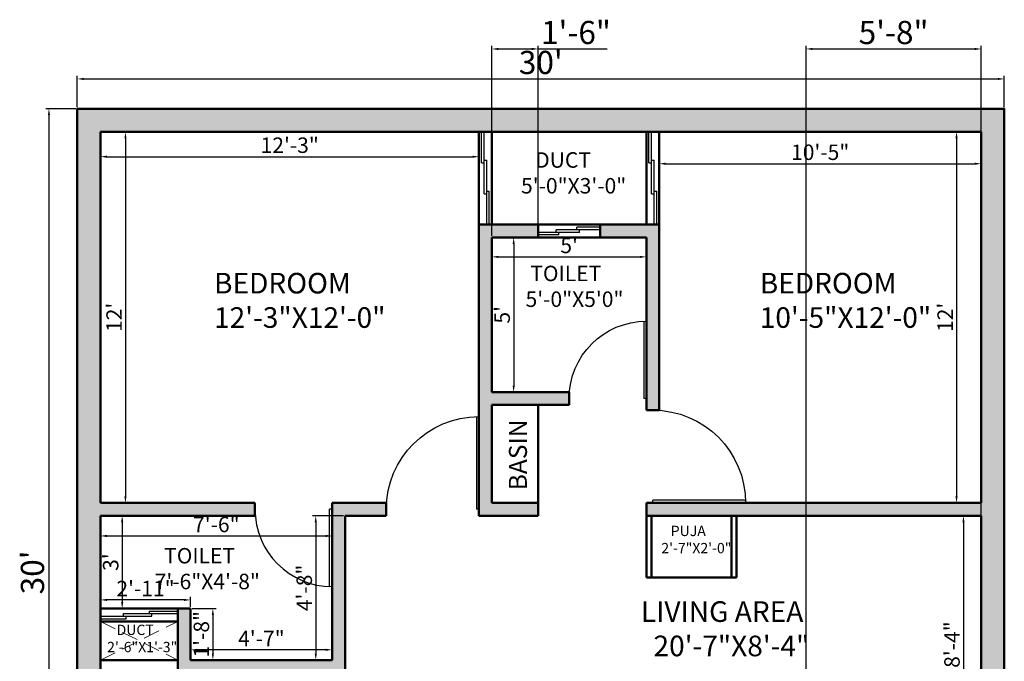
# Model space of a CAD drawing. Units: inches. Extents: x 3274 to 5176, y 1085 to 2172.
# Tile 2 of 16: x 3351 to 3733, y 1325 to 1574. Entities that reach past the tile are written whole.
import ezdxf

# ---------------------------------------------------------------- set-up
doc = ezdxf.new("R2010")
doc.units = ezdxf.units.IN
doc.linetypes.add('DASHED', pattern=[19.05, 12.7, -6.35])
for name, color, linetype, lineweight in [('A-ANNO-DIMS', 2, 'Continuous', 18), ('A-AREA-IDEN', 3, 'Continuous', 25), ('A-DOOR', 4, 'Continuous', 25), ('A-FLOR-OPEN', 7, 'DASHED', 18), ('A-GLAZ', 5, 'Continuous', 25), ('A-WALL', 7, 'Continuous', 50), ('A-WALL-PATT', 8, 'Continuous', 13)]:
    doc.layers.add(name, color=color, linetype=linetype, lineweight=lineweight)
doc.styles.get("Standard").update_dxf_attribs({"font": 'arial.ttf'})
doc.dimstyles.new('ISO-25', dxfattribs={"dimtxt": 9, "dimasz": 2.5, "dimexe": 1.25, "dimexo": 0.625, "dimtad": 1, "dimdec": 1, "dimlunit": 3, "dimtxsty": 'Standard', "dimcen": 2.5, "dimclrd": 4, "dimclre": 4, "dimclrt": 1, "dimadec": 0, "dimazin": 0, "dimtfac": 1, "dimtdec": 1, "dimtmove": 0, "dimatfit": 3, "dimfxl": 1, "dimarcsym": 0})

# ---------------------------------------------------------------- blocks, each defined once
blk = doc.blocks.new('1')
for p, q in [((0, 36), (0, 0)), ((1, 36), (1, 0)), ((0, 0), (1, 0))]:
    blk.add_line(p, q)
blk.add_arc((0, 0), 36, 0, 90)
blk = doc.blocks.new('2')
for p, q in [((0, 30), (0, 0)), ((1, 30), (1, 0)), ((0, 0), (1, 0))]:
    blk.add_line(p, q)
blk.add_arc((0, 0), 30, 0, 90)
blk = doc.blocks.new('*D10')
at = {"layer": 'A-ANNO-DIMS', "color": 0, "lineweight": -2, "transparency": 16777216}
for p, q in [((3373.3, 1539.91), (3373.3, 1552.09)), ((3375.8, 1550.84), (3730.8, 1550.84)), ((3733.3, 1539.91), (3733.3, 1552.09))]:
    blk.add_line(p, q, dxfattribs=at)
at = {"layer": 'A-ANNO-DIMS', "color": 0, "transparency": 16777216}
for points in [[(3375.8, 1551.26), (3375.8, 1550.43), (3373.3, 1550.84)], [(3730.8, 1551.26), (3730.8, 1550.43), (3733.3, 1550.84)]]:
    blk.add_solid(points, dxfattribs=at)
at = {"layer": 'Defpoints', "color": 0, "transparency": 16777216}
for p in [(3733.3, 1550.84), (3373.3, 1539.28), (3733.3, 1539.28)]:
    blk.add_point(p, dxfattribs=at)
at = {"layer": 'A-ANNO-DIMS', "color": 0, "transparency": 16777216, "insert": (3553.3, 1556.07), "char_height": 9, "attachment_point": 5}
blk.add_mtext("30'", dxfattribs=at)
blk = doc.blocks.new('*D11')
at = {"layer": 'A-ANNO-DIMS', "color": 0, "lineweight": -2, "transparency": 16777216}
for p, q in [((3372.68, 1539.28), (3361.05, 1539.28)), ((3362.3, 1536.78), (3362.3, 1181.78)), ((3372.68, 1179.28), (3361.05, 1179.28))]:
    blk.add_line(p, q, dxfattribs=at)
at = {"layer": 'A-ANNO-DIMS', "color": 0, "transparency": 16777216}
for points in [[(3361.88, 1536.78), (3362.71, 1536.78), (3362.3, 1539.28)], [(3361.88, 1181.78), (3362.71, 1181.78), (3362.3, 1179.28)]]:
    blk.add_solid(points, dxfattribs=at)
at = {"layer": 'Defpoints', "color": 0, "transparency": 16777216}
for p in [(3373.3, 1539.28), (3362.3, 1179.28), (3373.3, 1179.28)]:
    blk.add_point(p, dxfattribs=at)
at = {"layer": 'A-ANNO-DIMS', "color": 0, "transparency": 16777216, "insert": (3357.07, 1359.28), "char_height": 9, "attachment_point": 5, "rotation": 90}
blk.add_mtext("30'", dxfattribs=at)
blk = doc.blocks.new('*D12')
at = {"layer": 'A-ANNO-DIMS', "color": 0, "lineweight": -2, "transparency": 16777216}
for p, q in [((3382.3, 1529.66), (3382.3, 1519.4)), ((3529.3, 1529.66), (3529.3, 1519.4)), ((3384.8, 1520.65), (3526.8, 1520.65))]:
    blk.add_line(p, q, dxfattribs=at)
at = {"layer": 'A-ANNO-DIMS', "color": 0, "transparency": 16777216}
for points in [[(3384.8, 1521.07), (3384.8, 1520.24), (3382.3, 1520.65)], [(3526.8, 1521.07), (3526.8, 1520.24), (3529.3, 1520.65)]]:
    blk.add_solid(points, dxfattribs=at)
at = {"layer": 'Defpoints', "color": 0, "transparency": 16777216}
for p in [(3382.3, 1530.28), (3529.3, 1530.28), (3529.3, 1520.65)]:
    blk.add_point(p, dxfattribs=at)
at = {"layer": 'A-ANNO-DIMS', "color": 0, "transparency": 16777216, "insert": (3455.8, 1524.34), "char_height": 6, "attachment_point": 5}
blk.add_mtext('12\'-3"', dxfattribs=at)
blk = doc.blocks.new('*D13')
at = {"layer": 'A-ANNO-DIMS', "color": 0, "lineweight": -2, "transparency": 16777216}
for p, q in [((3382.93, 1530.28), (3393.26, 1530.28)), ((3392.01, 1527.78), (3392.01, 1388.78)), ((3382.93, 1386.28), (3393.26, 1386.28))]:
    blk.add_line(p, q, dxfattribs=at)
at = {"layer": 'A-ANNO-DIMS', "color": 0, "transparency": 16777216}
for points in [[(3391.59, 1527.78), (3392.42, 1527.78), (3392.01, 1530.28)], [(3391.59, 1388.78), (3392.42, 1388.78), (3392.01, 1386.28)]]:
    blk.add_solid(points, dxfattribs=at)
at = {"layer": 'Defpoints', "color": 0, "transparency": 16777216}
for p in [(3382.3, 1530.28), (3382.3, 1386.28), (3392.01, 1386.28)]:
    blk.add_point(p, dxfattribs=at)
at = {"layer": 'A-ANNO-DIMS', "color": 0, "transparency": 16777216, "insert": (3388.37, 1458.28), "char_height": 6, "attachment_point": 5, "rotation": 90}
blk.add_mtext("12'", dxfattribs=at)
blk = doc.blocks.new('*D14')
at = {"layer": 'A-ANNO-DIMS', "color": 0, "lineweight": -2, "transparency": 16777216}
for p, q in [((3417.3, 1325.91), (3417.3, 1330.49)), ((3469.8, 1329.24), (3419.8, 1329.24)), ((3472.3, 1325.91), (3472.3, 1330.49))]:
    blk.add_line(p, q, dxfattribs=at)
at = {"layer": 'A-ANNO-DIMS', "color": 0, "transparency": 16777216}
for points in [[(3419.8, 1329.65), (3419.8, 1328.82), (3417.3, 1329.24)], [(3469.8, 1329.65), (3469.8, 1328.82), (3472.3, 1329.24)]]:
    blk.add_solid(points, dxfattribs=at)
at = {"layer": 'Defpoints', "color": 0, "transparency": 16777216}
for p in [(3417.3, 1329.24), (3417.3, 1325.28), (3472.3, 1325.28)]:
    blk.add_point(p, dxfattribs=at)
at = {"layer": 'A-ANNO-DIMS', "color": 0, "transparency": 16777216, "insert": (3444.8, 1332.86), "char_height": 6, "attachment_point": 5}
blk.add_mtext('4\'-7"', dxfattribs=at)
blk = doc.blocks.new('*D15')
at = {"layer": 'A-ANNO-DIMS', "color": 0, "lineweight": -2, "transparency": 16777216}
for p, q in [((3382.93, 1381.28), (3391.99, 1381.28)), ((3390.74, 1378.78), (3390.74, 1347.78)), ((3382.93, 1345.28), (3391.99, 1345.28))]:
    blk.add_line(p, q, dxfattribs=at)
at = {"layer": 'A-ANNO-DIMS', "color": 0, "transparency": 16777216}
for points in [[(3390.32, 1378.78), (3391.16, 1378.78), (3390.74, 1381.28)], [(3390.32, 1347.78), (3391.16, 1347.78), (3390.74, 1345.28)]]:
    blk.add_solid(points, dxfattribs=at)
at = {"layer": 'Defpoints', "color": 0, "transparency": 16777216}
for p in [(3382.3, 1381.28), (3382.3, 1345.28), (3390.74, 1345.28)]:
    blk.add_point(p, dxfattribs=at)
at = {"layer": 'A-ANNO-DIMS', "color": 0, "transparency": 16777216, "insert": (3387.05, 1363.28), "char_height": 6, "attachment_point": 5, "rotation": 90}
blk.add_mtext("3'", dxfattribs=at)
blk = doc.blocks.new('*D16')
at = {"layer": 'A-ANNO-DIMS', "color": 0, "lineweight": -2, "transparency": 16777216}
for p, q in [((3382.3, 1380.66), (3382.3, 1372.19)), ((3472.3, 1380.66), (3472.3, 1372.19)), ((3384.8, 1373.44), (3469.8, 1373.44))]:
    blk.add_line(p, q, dxfattribs=at)
at = {"layer": 'A-ANNO-DIMS', "color": 0, "transparency": 16777216}
for points in [[(3384.8, 1373.86), (3384.8, 1373.02), (3382.3, 1373.44)], [(3469.8, 1373.86), (3469.8, 1373.02), (3472.3, 1373.44)]]:
    blk.add_solid(points, dxfattribs=at)
at = {"layer": 'Defpoints', "color": 0, "transparency": 16777216}
for p in [(3382.3, 1381.28), (3472.3, 1381.28), (3472.3, 1373.44)]:
    blk.add_point(p, dxfattribs=at)
at = {"layer": 'A-ANNO-DIMS', "color": 0, "transparency": 16777216, "insert": (3427.3, 1377.13), "char_height": 6, "attachment_point": 5}
blk.add_mtext('7\'-6"', dxfattribs=at)
blk = doc.blocks.new('*D17')
at = {"layer": 'A-ANNO-DIMS', "color": 0, "lineweight": -2, "transparency": 16777216}
for p, q in [((3417.93, 1345.28), (3427.21, 1345.28)), ((3425.96, 1342.78), (3425.96, 1327.78)), ((3417.93, 1325.28), (3427.21, 1325.28))]:
    blk.add_line(p, q, dxfattribs=at)
at = {"layer": 'A-ANNO-DIMS', "color": 0, "transparency": 16777216}
for points in [[(3425.54, 1342.78), (3426.37, 1342.78), (3425.96, 1345.28)], [(3425.54, 1327.78), (3426.37, 1327.78), (3425.96, 1325.28)]]:
    blk.add_solid(points, dxfattribs=at)
at = {"layer": 'Defpoints', "color": 0, "transparency": 16777216}
for p in [(3417.3, 1345.28), (3417.3, 1325.28), (3425.96, 1325.28)]:
    blk.add_point(p, dxfattribs=at)
at = {"layer": 'A-ANNO-DIMS', "color": 0, "transparency": 16777216, "insert": (3422.27, 1335.28), "char_height": 6, "attachment_point": 5, "rotation": 90}
blk.add_mtext('1\'-8"', dxfattribs=at)
blk = doc.blocks.new('*D18')
at = {"layer": 'A-ANNO-DIMS', "color": 0, "lineweight": -2, "transparency": 16777216}
for p, q in [((3382.3, 1345.91), (3382.3, 1349.86)), ((3417.3, 1345.91), (3417.3, 1349.86)), ((3414.8, 1348.61), (3384.8, 1348.61))]:
    blk.add_line(p, q, dxfattribs=at)
at = {"layer": 'A-ANNO-DIMS', "color": 0, "transparency": 16777216}
for points in [[(3384.8, 1349.02), (3384.8, 1348.19), (3382.3, 1348.61)], [(3414.8, 1349.02), (3414.8, 1348.19), (3417.3, 1348.61)]]:
    blk.add_solid(points, dxfattribs=at)
at = {"layer": 'Defpoints', "color": 0, "transparency": 16777216}
for p in [(3382.3, 1348.61), (3382.3, 1345.28), (3417.3, 1345.28)]:
    blk.add_point(p, dxfattribs=at)
at = {"layer": 'A-ANNO-DIMS', "color": 0, "transparency": 16777216, "insert": (3399.8, 1352.24), "char_height": 6, "attachment_point": 5}
blk.add_mtext('2\'-11"', dxfattribs=at)
blk = doc.blocks.new('*D19')
at = {"layer": 'A-ANNO-DIMS', "color": 0, "lineweight": -2, "transparency": 16777216}
for p, q in [((3476.68, 1381.28), (3464.66, 1381.28)), ((3465.91, 1378.78), (3465.91, 1327.78)), ((3471.68, 1325.28), (3464.66, 1325.28))]:
    blk.add_line(p, q, dxfattribs=at)
at = {"layer": 'A-ANNO-DIMS', "color": 0, "transparency": 16777216}
for points in [[(3465.5, 1378.78), (3466.33, 1378.78), (3465.91, 1381.28)], [(3465.5, 1327.78), (3466.33, 1327.78), (3465.91, 1325.28)]]:
    blk.add_solid(points, dxfattribs=at)
at = {"layer": 'Defpoints', "color": 0, "transparency": 16777216}
for p in [(3477.3, 1381.28), (3465.91, 1325.28), (3472.3, 1325.28)]:
    blk.add_point(p, dxfattribs=at)
at = {"layer": 'A-ANNO-DIMS', "color": 0, "transparency": 16777216, "insert": (3462.22, 1353.28), "char_height": 6, "attachment_point": 5, "rotation": 90}
blk.add_mtext('4\'-8"', dxfattribs=at)
blk = doc.blocks.new('*D28')
at = {"layer": 'A-ANNO-DIMS', "color": 0, "lineweight": -2, "transparency": 16777216}
for p, q in [((3723.68, 1381.28), (3716.2, 1381.28)), ((3717.45, 1378.78), (3717.45, 1283.78)), ((3723.68, 1281.28), (3716.2, 1281.28))]:
    blk.add_line(p, q, dxfattribs=at)
at = {"layer": 'A-ANNO-DIMS', "color": 0, "transparency": 16777216}
for points in [[(3717.03, 1378.78), (3717.86, 1378.78), (3717.45, 1381.28)], [(3717.03, 1283.78), (3717.86, 1283.78), (3717.45, 1281.28)]]:
    blk.add_solid(points, dxfattribs=at)
at = {"layer": 'Defpoints', "color": 0, "transparency": 16777216}
for p in [(3724.3, 1381.28), (3717.45, 1281.28), (3724.3, 1281.28)]:
    blk.add_point(p, dxfattribs=at)
at = {"layer": 'A-ANNO-DIMS', "color": 0, "transparency": 16777216, "insert": (3713.76, 1331.28), "char_height": 6, "attachment_point": 5, "rotation": 90}
blk.add_mtext('8\'-4"', dxfattribs=at)
blk = doc.blocks.new('*D30')
at = {"layer": 'A-ANNO-DIMS', "color": 0, "lineweight": -2, "transparency": 16777216}
for p, q in [((3599.3, 1529.66), (3599.3, 1516.67)), ((3724.3, 1529.66), (3724.3, 1516.67)), ((3601.8, 1517.92), (3721.8, 1517.92))]:
    blk.add_line(p, q, dxfattribs=at)
at = {"layer": 'A-ANNO-DIMS', "color": 0, "transparency": 16777216}
for points in [[(3601.8, 1518.34), (3601.8, 1517.51), (3599.3, 1517.92)], [(3721.8, 1518.34), (3721.8, 1517.51), (3724.3, 1517.92)]]:
    blk.add_solid(points, dxfattribs=at)
at = {"layer": 'Defpoints', "color": 0, "transparency": 16777216}
for p in [(3599.3, 1530.28), (3724.3, 1530.28), (3724.3, 1517.92)]:
    blk.add_point(p, dxfattribs=at)
at = {"layer": 'A-ANNO-DIMS', "color": 0, "transparency": 16777216, "insert": (3661.8, 1521.61), "char_height": 6, "attachment_point": 5}
blk.add_mtext('10\'-5"', dxfattribs=at)
blk = doc.blocks.new('*D31')
at = {"layer": 'A-ANNO-DIMS', "color": 0, "lineweight": -2, "transparency": 16777216}
for p, q in [((3723.68, 1530.28), (3713.49, 1530.28)), ((3714.74, 1527.78), (3714.74, 1388.78)), ((3723.68, 1386.28), (3713.49, 1386.28))]:
    blk.add_line(p, q, dxfattribs=at)
at = {"layer": 'A-ANNO-DIMS', "color": 0, "transparency": 16777216}
for points in [[(3714.32, 1527.78), (3715.16, 1527.78), (3714.74, 1530.28)], [(3714.32, 1388.78), (3715.16, 1388.78), (3714.74, 1386.28)]]:
    blk.add_solid(points, dxfattribs=at)
at = {"layer": 'Defpoints', "color": 0, "transparency": 16777216}
for p in [(3724.3, 1530.28), (3714.74, 1386.28), (3724.3, 1386.28)]:
    blk.add_point(p, dxfattribs=at)
at = {"layer": 'A-ANNO-DIMS', "color": 0, "transparency": 16777216, "insert": (3711.1, 1458.28), "char_height": 6, "attachment_point": 5, "rotation": 90}
blk.add_mtext("12'", dxfattribs=at)
blk = doc.blocks.new('*D32')
at = {"layer": 'A-ANNO-DIMS', "color": 0, "lineweight": -2, "transparency": 16777216}
for p, q in [((3534.3, 1488.66), (3534.3, 1480.52)), ((3594.3, 1488.66), (3594.3, 1480.52)), ((3536.8, 1481.77), (3591.8, 1481.77))]:
    blk.add_line(p, q, dxfattribs=at)
at = {"layer": 'A-ANNO-DIMS', "color": 0, "transparency": 16777216}
for points in [[(3536.8, 1482.18), (3536.8, 1481.35), (3534.3, 1481.77)], [(3591.8, 1482.18), (3591.8, 1481.35), (3594.3, 1481.77)]]:
    blk.add_solid(points, dxfattribs=at)
at = {"layer": 'Defpoints', "color": 0, "transparency": 16777216}
for p in [(3534.3, 1489.28), (3594.3, 1489.28), (3594.3, 1481.77)]:
    blk.add_point(p, dxfattribs=at)
at = {"layer": 'A-ANNO-DIMS', "color": 0, "transparency": 16777216, "insert": (3564.3, 1485.44), "char_height": 6, "attachment_point": 5}
blk.add_mtext("5'", dxfattribs=at)
blk = doc.blocks.new('*D33')
at = {"layer": 'A-ANNO-DIMS', "color": 0, "lineweight": -2, "transparency": 16777216}
for p, q in [((3534.93, 1489.28), (3544.02, 1489.28)), ((3542.77, 1486.78), (3542.77, 1431.78)), ((3534.93, 1429.28), (3544.02, 1429.28))]:
    blk.add_line(p, q, dxfattribs=at)
at = {"layer": 'A-ANNO-DIMS', "color": 0, "transparency": 16777216}
for points in [[(3542.35, 1486.78), (3543.18, 1486.78), (3542.77, 1489.28)], [(3542.35, 1431.78), (3543.18, 1431.78), (3542.77, 1429.28)]]:
    blk.add_solid(points, dxfattribs=at)
at = {"layer": 'Defpoints', "color": 0, "transparency": 16777216}
for p in [(3534.3, 1489.28), (3534.3, 1429.28), (3542.77, 1429.28)]:
    blk.add_point(p, dxfattribs=at)
at = {"layer": 'A-ANNO-DIMS', "color": 0, "transparency": 16777216, "insert": (3539.09, 1459.28), "char_height": 6, "attachment_point": 5, "rotation": 90}
blk.add_mtext("5'", dxfattribs=at)
blk = doc.blocks.new('WIN-24')
for p, q in [((4552.19, 1485.35), (4536.19, 1485.35)), ((4544.19, 1484.35), (4536.19, 1484.35)), ((4560.19, 1486.35), (4543.19, 1486.35)), ((4543.19, 1485.35), (4543.19, 1486.35)), ((4544.19, 1484.35), (4544.19, 1485.35)), ((4551.19, 1486.35), (4551.19, 1487.35)), ((4560.19, 1487.35), (4551.19, 1487.35)), ((4552.19, 1485.35), (4552.19, 1486.35))]:
    blk.add_line(p, q)
blk = doc.blocks.new('WIN-30')
for p, q in [((4366.19, 1316.35), (4386.19, 1316.35)), ((4366.19, 1315.35), (4376.19, 1315.35)), ((4375.19, 1317.35), (4396.19, 1317.35)), ((4375.19, 1316.35), (4375.19, 1317.35)), ((4376.19, 1315.35), (4376.19, 1316.35)), ((4385.19, 1318.35), (4396.19, 1318.35)), ((4385.19, 1317.35), (4385.19, 1318.35)), ((4386.19, 1316.35), (4386.19, 1317.35))]:
    blk.add_line(p, q)
blk = doc.blocks.new('WIN-36')
for p, q in [((4514.19, 1512.35), (4514.19, 1524.35)), ((4515.19, 1500.35), (4515.19, 1524.35)), ((4514.19, 1512.35), (4515.19, 1512.35)), ((4515.19, 1513.35), (4516.19, 1513.35)), ((4516.19, 1488.35), (4516.19, 1513.35)), ((4515.19, 1500.35), (4516.19, 1500.35)), ((4516.19, 1501.35), (4517.19, 1501.35)), ((4517.19, 1488.35), (4517.19, 1501.35))]:
    blk.add_line(p, q)
blk = doc.blocks.new('*D166')
at = {"layer": 'A-ANNO-DIMS', "color": 4, "lineweight": -2, "transparency": 16777216}
for p, q in [((3656.3, 1281.91), (3656.3, 1563.73)), ((3658.8, 1562.48), (3721.8, 1562.48)), ((3724.3, 1281.91), (3724.3, 1563.73))]:
    blk.add_line(p, q, dxfattribs=at)
at = {"layer": 'A-ANNO-DIMS', "color": 4, "transparency": 16777216}
for points in [[(3658.8, 1562.9), (3658.8, 1562.06), (3656.3, 1562.48)], [(3721.8, 1562.9), (3721.8, 1562.06), (3724.3, 1562.48)]]:
    blk.add_solid(points, dxfattribs=at)
at = {"layer": 'Defpoints', "color": 0, "transparency": 16777216}
for p in [(3724.3, 1562.48), (3656.3, 1281.28), (3724.3, 1281.28)]:
    blk.add_point(p, dxfattribs=at)
at = {"layer": 'A-ANNO-DIMS', "color": 1, "transparency": 16777216, "insert": (3690.3, 1567.7), "char_height": 9, "attachment_point": 5}
blk.add_mtext('5\'-8"', dxfattribs=at)
blk = doc.blocks.new('*D167')
at = {"layer": 'A-ANNO-DIMS', "color": 4, "lineweight": -2, "transparency": 16777216}
for p, q in [((3534.3, 1489.91), (3534.3, 1563.73)), ((3536.8, 1562.48), (3549.8, 1562.48)), ((3552.3, 1489.91), (3552.3, 1563.73)), ((3552.3, 1562.48), (3579.13, 1562.48))]:
    blk.add_line(p, q, dxfattribs=at)
at = {"layer": 'A-ANNO-DIMS', "color": 4, "transparency": 16777216}
for points in [[(3536.8, 1562.9), (3536.8, 1562.06), (3534.3, 1562.48)], [(3549.8, 1562.9), (3549.8, 1562.06), (3552.3, 1562.48)]]:
    blk.add_solid(points, dxfattribs=at)
at = {"layer": 'Defpoints', "color": 0, "transparency": 16777216}
for p in [(3552.3, 1562.48), (3534.3, 1489.28), (3552.3, 1489.28)]:
    blk.add_point(p, dxfattribs=at)
at = {"layer": 'A-ANNO-DIMS', "color": 1, "transparency": 16777216, "insert": (3566.96, 1567.7), "char_height": 9, "attachment_point": 5}
blk.add_mtext('1\'-6"', dxfattribs=at)

msp = doc.modelspace()

# ---------------------------------------------------------------- hatches: boundary and pattern name
at = {"layer": 'A-WALL-PATT'}
h = msp.add_hatch(color=256, dxfattribs=at)
h.dxf.hatch_style = 1
h.paths.add_polyline_path([(3733.3, 1539.28), (3373.3, 1539.28), (3373.3, 1179.28), (3406.3, 1179.28), (3406.3, 1188.28), (3382.3, 1188.28), (3382.3, 1272.28), (3442.3, 1272.28), (3442.3, 1277.28), (3382.3, 1277.28), (3382.3, 1381.28), (3442.3, 1381.28), (3442.3, 1386.28), (3382.3, 1386.28), (3382.3, 1530.28), (3724.3, 1530.28), (3724.3, 1386.28), (3594.3, 1386.28), (3594.3, 1381.28), (3724.3, 1381.28), (3724.3, 1281.28), (3656.3, 1281.28), (3656.3, 1272.28), (3724.3, 1272.28), (3724.3, 1188.28), (3682.3, 1188.28), (3682.3, 1179.28), (3733.3, 1179.28)])
h.paths.add_polyline_path([(3477.3, 1381.28), (3493.3, 1381.28), (3493.3, 1386.28), (3472.3, 1386.28), (3472.3, 1325.28), (3417.3, 1325.28), (3417.3, 1345.28), (3412.3, 1345.28), (3412.3, 1320.28), (3472.3, 1320.28), (3472.3, 1272.28), (3493.3, 1272.28), (3493.3, 1277.28), (3477.3, 1277.28)], flags=17)
h.paths.add_polyline_path([(3534.3, 1489.28), (3552.3, 1489.28), (3552.3, 1494.28), (3529.3, 1494.28), (3529.3, 1381.28), (3552.3, 1381.28), (3552.3, 1386.28), (3534.3, 1386.28), (3534.3, 1424.28), (3564.3, 1424.28), (3564.3, 1429.28), (3534.3, 1429.28)], flags=17)
h.paths.add_polyline_path([(3599.3, 1494.28), (3576.3, 1494.28), (3576.3, 1489.28), (3594.3, 1489.28), (3594.3, 1422.28), (3599.3, 1422.28)], flags=17)
h.paths.add_polyline_path([(3534.3, 1272.28), (3539.3, 1272.28), (3539.3, 1281.28), (3529.3, 1281.28), (3529.3, 1188.28), (3478.3, 1188.28), (3478.3, 1179.28), (3534.3, 1179.28)], flags=17)
h.paths.add_polyline_path([(3596.3, 1281.28), (3587.3, 1281.28), (3587.3, 1276.78), (3587.3, 1272.28), (3596.3, 1272.28)], flags=17)
h.paths.add_polyline_path([(3610.3, 1188.28), (3594.3, 1188.28), (3594.3, 1179.28), (3610.3, 1179.28)], flags=17)
h.paths.add_polyline_path([(3589.35, 1322.21), (3663.55, 1322.21), (3663.55, 1352.06), (3589.35, 1352.06)], flags=25)
h.paths.add_polyline_path([(3545.54, 1458.93), (3584.72, 1458.93), (3584.72, 1481.32), (3545.54, 1481.32)], flags=25)
h.paths.add_polyline_path([(3635.11, 1449.68), (3703.51, 1449.68), (3703.51, 1479.54), (3635.11, 1479.54)], flags=25)
h.paths.add_polyline_path([(3543.78, 1502.97), (3585.75, 1502.97), (3585.75, 1525.36), (3543.78, 1525.36)], flags=25)
h.paths.add_polyline_path([(3423.19, 1449.68), (3491.58, 1449.68), (3491.58, 1479.54), (3423.19, 1479.54)], flags=25)

# ---------------------------------------------------------------- linework, layer by layer
at = {"layer": 'A-FLOR-OPEN', "ltscale": 0.5}
for p, q in [((3382.3, 1340.28), (3412.3, 1325.28)), ((3382.3, 1325.28), (3412.3, 1340.28))]:
    msp.add_line(p, q, dxfattribs=at)
at = {"layer": 'A-WALL'}
for p, q in [((3382.3, 1530.28), (3724.3, 1530.28)), ((3382.3, 1386.28), (3382.3, 1530.28)), ((3529.3, 1381.28), (3529.3, 1530.28)), ((3534.3, 1494.28), (3534.3, 1530.28)), ((3594.3, 1530.28), (3594.3, 1494.28)), ((3599.3, 1530.28), (3599.3, 1422.28)), ((3724.3, 1530.28), (3724.3, 1386.28)), ((3529.3, 1494.28), (3599.3, 1494.28)), ((3552.3, 1489.28), (3552.3, 1494.28)), ((3576.3, 1489.28), (3576.3, 1494.28)), ((3534.3, 1489.28), (3594.3, 1489.28)), ((3534.3, 1429.28), (3534.3, 1489.28)), ((3594.3, 1489.28), (3594.3, 1422.28)), ((3534.3, 1429.28), (3564.3, 1429.28)), ((3564.3, 1429.28), (3564.3, 1424.28)), ((3534.3, 1424.28), (3564.3, 1424.28)), ((3534.3, 1386.28), (3534.3, 1424.28)), ((3552.3, 1381.28), (3552.3, 1424.28)), ((3594.3, 1422.28), (3599.3, 1422.28)), ((3382.3, 1386.28), (3442.3, 1386.28)), ((3442.3, 1381.28), (3442.3, 1386.28)), ((3472.3, 1386.28), (3493.3, 1386.28)), ((3472.3, 1325.28), (3472.3, 1386.28)), ((3493.3, 1381.28), (3493.3, 1386.28)), ((3534.3, 1386.28), (3552.3, 1386.28)), ((3594.3, 1386.28), (3724.3, 1386.28)), ((3594.3, 1386.28), (3594.3, 1357.28)), ((3382.3, 1381.28), (3442.3, 1381.28)), ((3382.3, 1277.28), (3382.3, 1381.28)), ((3477.3, 1381.28), (3493.3, 1381.28)), ((3477.3, 1277.28), (3477.3, 1381.28)), ((3529.3, 1381.28), (3552.3, 1381.28)), ((3594.3, 1381.28), (3724.3, 1381.28)), ((3596.3, 1381.28), (3596.3, 1357.28)), ((3627.3, 1381.28), (3627.3, 1357.28)), ((3629.3, 1381.28), (3629.3, 1357.28)), ((3724.3, 1381.28), (3724.3, 1281.28)), ((3594.3, 1357.28), (3629.3, 1357.28)), ((3382.3, 1345.28), (3417.3, 1345.28)), ((3412.3, 1320.28), (3412.3, 1345.28)), ((3417.3, 1325.28), (3417.3, 1345.28)), ((3382.3, 1340.28), (3412.3, 1340.28)), ((3382.3, 1325.28), (3412.3, 1325.28)), ((3417.3, 1325.28), (3472.3, 1325.28))]:
    msp.add_line(p, q, dxfattribs=at)
msp.add_lwpolyline([(3534.3, 1179.28), (3373.3, 1179.28), (3373.3, 1539.28), (3733.3, 1539.28), (3733.3, 1179.28), (3594.3, 1179.28)], dxfattribs=at)

# ---------------------------------------------------------------- block references
at = {"layer": 'A-DOOR', "xscale": -1}
for name, p in [('2', (3594.3, 1426.78)), ('1', (3529.3, 1383.78))]:
    msp.add_blockref(name, p, dxfattribs=at)
at = {"layer": 'A-DOOR', "xscale": -1, "rotation": 270}
msp.add_blockref('1', (3596.8, 1386.28), dxfattribs=at)
at = {"layer": 'A-DOOR', "rotation": 180}
msp.add_blockref('2', (3472.3, 1383.78), dxfattribs=at)
at = {"layer": 'A-GLAZ'}
for name, p in [('WIN-36', (-983.89, 5.93)), ('WIN-36', (-918.89, 5.93)), ('WIN-24', (-983.89, 5.93)), ('WIN-30', (-983.89, 25.93))]:
    msp.add_blockref(name, p, dxfattribs=at)

# ---------------------------------------------------------------- texts
at = {"layer": 'A-AREA-IDEN', "attachment_point": 1}
for s, width, heights, insert, char_height in [('   DUCT\\P5\'-0"X3\'-0"', 58.0121, [16.24], (3545.63, 1522.37), 6), (' TOILET\\P5\'-0"X5\'0"', 58.0121, [0], (3547.39, 1478.34), 6), ('BEDROOM\\P12\'-3"X12\'-0"', 58.0121, [0], (3426.41, 1475.56), 8), ('BEDROOM\\P10\'-5"X12\'-0"', 58.0121, [0], (3638.33, 1475.56), 8), ('   PUJA\\P2\'-7"X2\'-0"', 58.0121, [16.24], (3600.1, 1377.39), 4), ('  TOILET\\P7\'-6"X4\'-8"', 58.0121, [16.24], (3403.37, 1368.76), 6), ('LIVING AREA\\P  20\'-7"X8\'-4"', 90.1483, [0], (3592.17, 1348.08), 8), ('   DUCT\\P2\'-6"X1\'-3"', 58.0121, [16.24], (3384.9, 1338.99), 4)]:
    msp.add_mtext_dynamic_manual_height_columns(s, width=width, gutter_width=30, heights=heights, dxfattribs=dict(at, insert=insert, char_height=char_height))
at = {"layer": 'A-AREA-IDEN', "insert": (3540.92, 1391.17), "char_height": 7, "attachment_point": 1, "rotation": 90}
msp.add_mtext_dynamic_manual_height_columns('BASIN', width=147.1149, gutter_width=30, heights=[0], dxfattribs=at)

# ---------------------------------------------------------------- dimensions: what is measured, and where the dimension line sits
at = {"layer": 'A-ANNO-DIMS'}
for base, p1, p2, override, picture, middle in [((3552.3, 1562.48), (3534.3, 1489.28), (3552.3, 1489.28), {"dimdec": 1, "dimlfac": 1, "dimrnd": 0, "dimzin": 1, "dimdsep": 46, "dimlunit": 4, "dimfrac": 2}, '*D167', (3566.96, 1567.7)), ((3724.3, 1562.48), (3656.3, 1281.28), (3724.3, 1281.28), {"dimdec": 1, "dimlfac": 1, "dimrnd": 0, "dimzin": 1, "dimdsep": 46, "dimlunit": 4, "dimfrac": 2}, '*D166', (3690.3, 1567.7)), ((3733.3, 1550.84), (3373.3, 1539.28), (3733.3, 1539.28), {"dimclrd": 0, "dimclre": 0, "dimclrt": 0}, '*D10', (3553.3, 1556.07)), ((3529.3, 1520.65), (3382.3, 1530.28), (3529.3, 1530.28), {"dimtxt": 6, "dimclrd": 0, "dimclre": 0, "dimclrt": 0}, '*D12', (3455.8, 1524.34)), ((3724.3, 1517.92), (3599.3, 1530.28), (3724.3, 1530.28), {"dimtxt": 6, "dimclrd": 0, "dimclre": 0, "dimclrt": 0}, '*D30', (3661.8, 1521.61)), ((3594.3, 1481.77), (3534.3, 1489.28), (3594.3, 1489.28), {"dimtxt": 6, "dimclrd": 0, "dimclre": 0, "dimclrt": 0}, '*D32', (3564.3, 1485.44)), ((3472.3, 1373.44), (3382.3, 1381.28), (3472.3, 1381.28), {"dimtxt": 6, "dimclrd": 0, "dimclre": 0, "dimclrt": 0}, '*D16', (3427.3, 1377.13)), ((3382.3, 1348.61), (3417.3, 1345.28), (3382.3, 1345.28), {"dimtxt": 6, "dimclrd": 0, "dimclre": 0, "dimclrt": 0}, '*D18', (3399.8, 1352.24)), ((3417.3, 1329.24), (3472.3, 1325.28), (3417.3, 1325.28), {"dimtxt": 6, "dimclrd": 0, "dimclre": 0, "dimclrt": 0}, '*D14', (3444.8, 1332.86))]:
    dim = msp.add_linear_dim(base=base, p1=p1, p2=p2, dimstyle='ISO-25', override=override, dxfattribs=at)
    dim.commit()
    dim.dimension.update_dxf_attribs({"geometry": picture, "text_midpoint": middle})
for base, p1, p2, override, picture, middle in [((3362.3, 1179.28), (3373.3, 1539.28), (3373.3, 1179.28), {"dimclrd": 0, "dimclre": 0, "dimclrt": 0}, '*D11', (3357.07, 1359.28)), ((3392.01, 1386.28), (3382.3, 1530.28), (3382.3, 1386.28), {"dimtxt": 6, "dimclrd": 0, "dimclre": 0, "dimclrt": 0}, '*D13', (3388.37, 1458.28)), ((3714.74, 1386.28), (3724.3, 1530.28), (3724.3, 1386.28), {"dimtxt": 6, "dimclrd": 0, "dimclre": 0, "dimclrt": 0}, '*D31', (3711.1, 1458.28)), ((3542.77, 1429.28), (3534.3, 1489.28), (3534.3, 1429.28), {"dimtxt": 6, "dimclrd": 0, "dimclre": 0, "dimclrt": 0}, '*D33', (3539.09, 1459.28)), ((3390.74, 1345.28), (3382.3, 1381.28), (3382.3, 1345.28), {"dimtxt": 6, "dimclrd": 0, "dimclre": 0, "dimclrt": 0}, '*D15', (3387.05, 1363.28)), ((3465.91, 1325.28), (3477.3, 1381.28), (3472.3, 1325.28), {"dimtxt": 6, "dimclrd": 0, "dimclre": 0, "dimclrt": 0}, '*D19', (3462.22, 1353.28)), ((3717.45, 1281.28), (3724.3, 1381.28), (3724.3, 1281.28), {"dimtxt": 6, "dimclrd": 0, "dimclre": 0, "dimclrt": 0}, '*D28', (3713.76, 1331.28)), ((3425.96, 1325.28), (3417.3, 1345.28), (3417.3, 1325.28), {"dimtxt": 6, "dimclrd": 0, "dimclre": 0, "dimclrt": 0}, '*D17', (3422.27, 1335.28))]:
    dim = msp.add_linear_dim(base=base, p1=p1, p2=p2, angle=90, dimstyle='ISO-25', override=override, dxfattribs=at)
    dim.commit()
    dim.dimension.update_dxf_attribs({"geometry": picture, "text_midpoint": middle})

doc.saveas('drawing.dxf')
